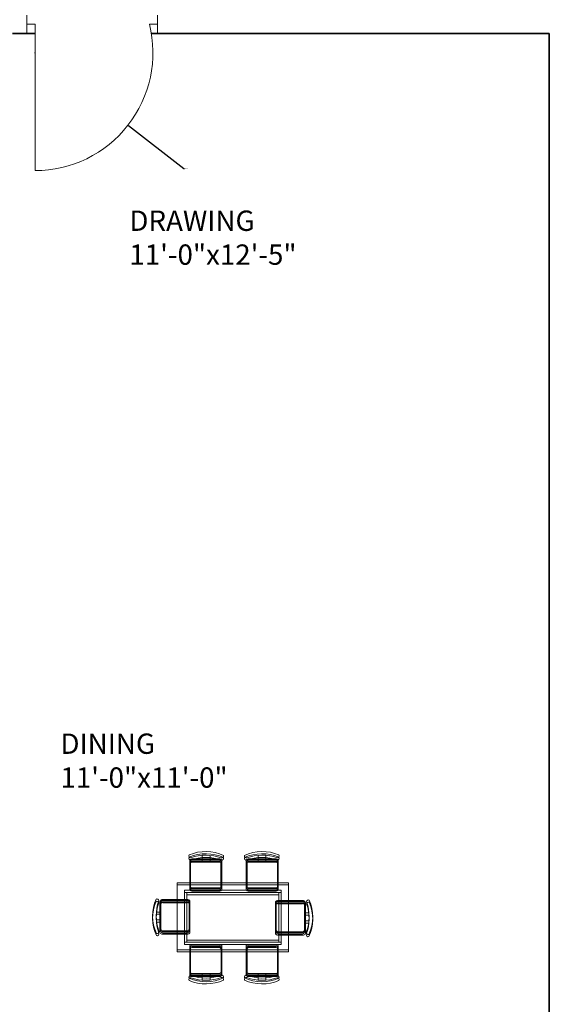
# Model space of a CAD drawing. Units: inches. Extents: x 2163 to 2982, y 1024 to 2288.
# Tile 4 of 22: x 2452 to 2582, y 1395 to 1637. Entities that reach past the tile are written whole.
import ezdxf

# ---------------------------------------------------------------- set-up
doc = ezdxf.new("R2010")
doc.units = ezdxf.units.IN
for name, color, linetype, lineweight in [('A-ANNO-DIMS', 2, 'Continuous', 18), ('A-AREA-IDEN', 7, 'Continuous', 18), ('A-DOOR', 11, 'Continuous', 18), ('A-FURN', 8, 'Continuous', 13), ('A-WALL', 7, 'Continuous', 35)]:
    doc.layers.add(name, color=color, linetype=linetype, lineweight=lineweight)
doc.styles.get("Standard").update_dxf_attribs({"font": 'arial.ttf'})
doc.dimstyles.get("Standard").update_dxf_attribs({"dimtxt": 0.18, "dimasz": 0.18, "dimexe": 0.18, "dimexo": 0.0625, "dimgap": 0.09, "dimtad": 0, "dimtih": 1, "dimtoh": 1, "dimdec": 4, "dimzin": 0, "dimdsep": 46, "dimtxsty": 'Standard', "dimcen": 0.09, "dimadec": 0, "dimazin": 0, "dimtfac": 1, "dimtdec": 4, "dimtofl": 0, "dimtmove": 0, "dimatfit": 3, "dimfxl": 1, "dimtolj": 1, "dimtzin": 0, "dimarcsym": 0})

# ---------------------------------------------------------------- blocks, each defined once
blk = doc.blocks.new('TABLE-DINING')
for points in [[(0, 17.02), (27.45, 17.02), (27.45, 0.55), (0, 0.55)], [(0, 17.02), (27.45, 17.02), (27.45, 0.55), (0, 0.55)], [(0, 17.02), (27.45, 17.02), (27.45, 0.55), (0, 0.55)], [(0, 17.02), (27.45, 17.02), (27.45, 0.55), (0, 0.55)], [(0, 16.47), (27.45, 16.47), (27.45, 0), (0, 0)], [(0, 16.47), (27.45, 16.47), (27.45, 0), (0, 0)], [(0, 16.47), (27.45, 16.47), (27.45, 0), (0, 0)], [(0, 16.47), (27.45, 16.47), (27.45, 0), (0, 0)], [(1.83, 15.19), (25.62, 15.19), (25.62, 2.38), (1.83, 2.38)], [(1.83, 15.19), (25.62, 15.19), (25.62, 2.38), (1.83, 2.38)], [(1.83, 15.19), (25.62, 15.19), (25.62, 2.38), (1.83, 2.38)], [(1.83, 15.19), (25.62, 15.19), (25.62, 2.38), (1.83, 2.38)], [(1.83, 14.64), (25.62, 14.64), (25.62, 1.83), (1.83, 1.83)], [(1.83, 14.64), (25.62, 14.64), (25.62, 1.83), (1.83, 1.83)], [(1.83, 14.64), (25.62, 14.64), (25.62, 1.83), (1.83, 1.83)], [(1.83, 14.64), (25.62, 14.64), (25.62, 1.83), (1.83, 1.83)], [(2.38, 14.64), (25.07, 14.64), (25.07, 2.93), (2.38, 2.93)], [(2.38, 14.64), (25.07, 14.64), (25.07, 2.93), (2.38, 2.93)], [(2.38, 14.64), (25.07, 14.64), (25.07, 2.93), (2.38, 2.93)], [(2.38, 14.64), (25.07, 14.64), (25.07, 2.93), (2.38, 2.93)], [(2.38, 14.09), (25.07, 14.09), (25.07, 2.38), (2.38, 2.38)], [(2.38, 14.09), (25.07, 14.09), (25.07, 2.38), (2.38, 2.38)], [(2.38, 14.09), (25.07, 14.09), (25.07, 2.38), (2.38, 2.38)], [(2.38, 14.09), (25.07, 14.09), (25.07, 2.38), (2.38, 2.38)]]:
    blk.add_lwpolyline(points, close=True)
blk = doc.blocks.new('CHAIR-DINING-A')
for points in [[(0.45, 8.2, -0.175809), (7.92, 8.14, 0.578392), (8.49, 8.77, 0.214524), (0.05, 8.88, 0.552014), (0.45, 8.2, -0.065079)], [(0.45, 8.2, -0.175809), (7.92, 8.14, 0.578392), (8.49, 8.77, 0.214524), (0.05, 8.88, 0.552014), (0.45, 8.2, -0.065079)], [(0.45, 8.2, -0.175809), (7.92, 8.14, 0.578392), (8.49, 8.77, 0.214524), (0.05, 8.88, 0.552014), (0.45, 8.2, -0.065079)], [(0.45, 8.2, -0.175809), (7.92, 8.14, 0.578392), (8.49, 8.77, 0.214524), (0.05, 8.88, 0.552014), (0.45, 8.2, -0.065079)], [(0.45, 7.65, -0.175809), (7.92, 7.6, 0.578392), (8.49, 8.22, 0.214524), (0.05, 8.33, 0.552014), (0.45, 7.65, -0.065079)], [(0.45, 7.65, -0.175809), (7.92, 7.6, 0.578392), (8.49, 8.22, 0.214524), (0.05, 8.33, 0.552014), (0.45, 7.65, -0.065079)], [(0.45, 7.65, -0.175809), (7.92, 7.6, 0.578392), (8.49, 8.22, 0.214524), (0.05, 8.33, 0.552014), (0.45, 7.65, -0.065079)], [(0.45, 7.65, -0.175809), (7.92, 7.6, 0.578392), (8.49, 8.22, 0.214524), (0.05, 8.33, 0.552014), (0.45, 7.65, -0.065079)], [(7.61, 7.9), (0.67, 7.9, 0.414214), (0.18, 7.42), (0.18, 1.03, 0.414214), (0.67, 0.55), (7.61, 0.55, 0.414214), (8.09, 1.03), (8.09, 7.42, 0.414214), (7.61, 7.9)], [(7.61, 7.9), (0.67, 7.9, 0.414214), (0.18, 7.42), (0.18, 1.03, 0.414214), (0.67, 0.55), (7.61, 0.55, 0.414214), (8.09, 1.03), (8.09, 7.42, 0.414214), (7.61, 7.9)], [(7.61, 7.9), (0.67, 7.9, 0.414214), (0.18, 7.42), (0.18, 1.03, 0.414214), (0.67, 0.55), (7.61, 0.55, 0.414214), (8.09, 1.03), (8.09, 7.42, 0.414214), (7.61, 7.9)], [(7.61, 7.9), (0.67, 7.9, 0.414214), (0.18, 7.42), (0.18, 1.03, 0.414214), (0.67, 0.55), (7.61, 0.55, 0.414214), (8.09, 1.03), (8.09, 7.42, 0.414214), (7.61, 7.9)], [(7.61, 7.35), (0.67, 7.35, 0.414214), (0.18, 6.87), (0.18, 0.49, 0.414214), (0.67, 0), (7.61, 0, 0.414214), (8.09, 0.49), (8.09, 6.87, 0.414214), (7.61, 7.35)], [(7.61, 7.35), (0.67, 7.35, 0.414214), (0.18, 6.87), (0.18, 0.49, 0.414214), (0.67, 0), (7.61, 0, 0.414214), (8.09, 0.49), (8.09, 6.87, 0.414214), (7.61, 7.35)], [(7.61, 7.35), (0.67, 7.35, 0.414214), (0.18, 6.87), (0.18, 0.49, 0.414214), (0.67, 0), (7.61, 0, 0.414214), (8.09, 0.49), (8.09, 6.87, 0.414214), (7.61, 7.35)], [(7.61, 7.35), (0.67, 7.35, 0.414214), (0.18, 6.87), (0.18, 0.49, 0.414214), (0.67, 0), (7.61, 0, 0.414214), (8.09, 0.49), (8.09, 6.87, 0.414214), (7.61, 7.35)], [(5.17, 7.9), (5.17, 8.78, -0.064759)], [(5.17, 7.9), (5.17, 8.78, -0.064759)], [(5.17, 7.9), (5.17, 8.78, -0.064759)], [(5.17, 7.9), (5.17, 8.78, -0.064759)], [(5.17, 7.35), (5.17, 8.23, -0.064759)], [(5.17, 7.35), (5.17, 8.23, -0.064759)], [(5.17, 7.35), (5.17, 8.23, -0.064759)], [(5.17, 7.35), (5.17, 8.23, -0.064759)]]:
    blk.add_lwpolyline(points, format="xyb")
for points in [[(0.67, 7.68), (7.39, 7.68, -0.414214), (7.87, 7.2), (7.87, 1.25, -0.414214), (7.39, 0.77), (0.67, 0.77, -0.512069), (0.4, 1.25), (0.4, 7.2, -0.512069)], [(0.67, 7.68), (7.39, 7.68, -0.414214), (7.87, 7.2), (7.87, 1.25, -0.414214), (7.39, 0.77), (0.67, 0.77, -0.512069), (0.4, 1.25), (0.4, 7.2, -0.512069)], [(0.67, 7.68), (7.39, 7.68, -0.414214), (7.87, 7.2), (7.87, 1.25, -0.414214), (7.39, 0.77), (0.67, 0.77, -0.512069), (0.4, 1.25), (0.4, 7.2, -0.512069)], [(0.67, 7.68), (7.39, 7.68, -0.414214), (7.87, 7.2), (7.87, 1.25, -0.414214), (7.39, 0.77), (0.67, 0.77, -0.512069), (0.4, 1.25), (0.4, 7.2, -0.512069)], [(0.67, 7.13), (7.39, 7.13, -0.414214), (7.87, 6.65), (7.87, 0.7, -0.414214), (7.39, 0.22), (0.67, 0.22, -0.512069), (0.4, 0.7), (0.4, 6.65, -0.512069)], [(0.67, 7.13), (7.39, 7.13, -0.414214), (7.87, 6.65), (7.87, 0.7, -0.414214), (7.39, 0.22), (0.67, 0.22, -0.512069), (0.4, 0.7), (0.4, 6.65, -0.512069)], [(0.67, 7.13), (7.39, 7.13, -0.414214), (7.87, 6.65), (7.87, 0.7, -0.414214), (7.39, 0.22), (0.67, 0.22, -0.512069), (0.4, 0.7), (0.4, 6.65, -0.512069)], [(0.67, 7.13), (7.39, 7.13, -0.414214), (7.87, 6.65), (7.87, 0.7, -0.414214), (7.39, 0.22), (0.67, 0.22, -0.512069), (0.4, 0.7), (0.4, 6.65, -0.512069)]]:
    blk.add_lwpolyline(points, format="xyb", close=True)
for points in [[(3.23, 8.8), (3.23, 7.9)], [(3.23, 8.8), (3.23, 7.9)], [(3.23, 8.79), (3.23, 7.9)], [(3.23, 8.79), (3.23, 7.9)], [(3.23, 8.25), (3.23, 7.35)], [(3.23, 8.25), (3.23, 7.35)], [(3.23, 8.25), (3.23, 7.35)], [(3.23, 8.25), (3.23, 7.35)]]:
    blk.add_lwpolyline(points)
blk = doc.blocks.new('*D43')
at = {"layer": 'A-ANNO-DIMS', "color": 0, "lineweight": -2, "transparency": 16777216}
for p, q in [((2455.83, 1628.97), (2456.01, 1628.97)), ((2455.92, 1628.88), (2455.92, 1629.06)), ((2492.45, 1600.48), (2478.89, 1611.05)), ((2492.63, 1600.48), (2492.45, 1600.48))]:
    blk.add_line(p, q, dxfattribs=at)
at = {"layer": 'A-ANNO-DIMS', "color": 0, "transparency": 16777216}
blk.add_solid([(2478.91, 1611.08), (2478.87, 1611.03), (2478.75, 1611.16)], dxfattribs=at)
at = {"layer": 'Defpoints', "color": 0, "transparency": 16777216}
for p in [(2455.92, 1628.97), (2478.75, 1611.16)]:
    blk.add_point(p, dxfattribs=at)
at = {"layer": 'A-ANNO-DIMS', "color": 0, "transparency": 16777216, "insert": (2493.11, 1600.48), "char_height": 0.18, "attachment_point": 5}
blk.add_mtext('\\A1;R28.95', dxfattribs=at)

msp = doc.modelspace()

# ---------------------------------------------------------------- linework, layer by layer
at = {"layer": 'A-DOOR'}
for p, q in [((2453.9219, 1633.7688), (2453.9219, 1638.2688)), ((2453.9219, 1638.2688), (2453.9219, 1636.0188)), ((2486.0038, 1638.2688), (2486.0038, 1633.7688)), ((2453.9219, 1636.0188), (2455.9219, 1636.0188)), ((2455.9219, 1636.0188), (2455.9219, 1600.0188)), ((2486.0038, 1636.0188), (2484.0038, 1636.0188)), ((2486.0038, 1633.7688), (2486.0038, 1636.0188))]:
    msp.add_line(p, q, dxfattribs=at)
msp.add_arc((2455.9219, 1628.9716), 28.9527, 270, 14.087641, dxfattribs=at)
at = {"layer": 'A-FURN'}
for points in [[(2507.9678, 1430.974, -0.57839206), (2507.4014, 1431.5967, -0.21452438), (2515.8396, 1431.7099, -0.55201397), (2515.4432, 1431.0306, 0.1758092), (2507.9678, 1430.974)], [(2507.9678, 1430.974, -0.57839206), (2507.4014, 1431.5967, -0.21452438), (2515.8396, 1431.7099, -0.55201397), (2515.4432, 1431.0306, 0.1758092), (2507.9678, 1430.974)], [(2507.9678, 1430.9737, -0.57839206), (2507.4015, 1431.5964, -0.21452438), (2515.8396, 1431.7096, -0.55201397), (2515.4432, 1431.0303, 0.1758092), (2507.9678, 1430.9737)], [(2507.9678, 1430.9737, -0.57839206), (2507.4015, 1431.5964, -0.21452438), (2515.8396, 1431.7096, -0.55201397), (2515.4432, 1431.0303, 0.1758092), (2507.9678, 1430.9737)], [(2507.9678, 1430.4251, -0.57839206), (2507.4014, 1431.0478, -0.21452438), (2515.8396, 1431.161, -0.55201397), (2515.4432, 1430.4817, 0.1758092), (2507.9678, 1430.4251)], [(2507.9678, 1430.4251, -0.57839206), (2507.4014, 1431.0478, -0.21452438), (2515.8396, 1431.161, -0.55201397), (2515.4432, 1430.4817, 0.1758092), (2507.9678, 1430.4251)], [(2507.9678, 1430.4248, -0.57839206), (2507.4015, 1431.0475, -0.21452438), (2515.8396, 1431.1607, -0.55201397), (2515.4432, 1430.4814, 0.1758092), (2507.9678, 1430.4248)], [(2507.9678, 1430.4248, -0.57839206), (2507.4015, 1431.0475, -0.21452438), (2515.8396, 1431.1607, -0.55201397), (2515.4432, 1430.4814, 0.1758092), (2507.9678, 1430.4248)], [(2510.7226, 1430.7306), (2510.7226, 1431.6082, 0.06475861)], [(2510.7226, 1430.7306), (2510.7226, 1431.6082, 0.06475861)], [(2510.7226, 1430.7303), (2510.7226, 1431.608, 0.06475861)], [(2510.7226, 1430.7303), (2510.7226, 1431.608, 0.06475861)], [(2515.2249, 1430.7306, -0.41421356), (2515.7104, 1430.245), (2515.7104, 1423.8639, -0.41421356), (2515.2249, 1423.3784), (2508.2849, 1423.3784, -0.41421356), (2507.7994, 1423.8639), (2507.7994, 1430.245, -0.41421356), (2508.2849, 1430.7306), (2515.2249, 1430.7306)], [(2515.2249, 1430.7306, -0.41421356), (2515.7104, 1430.245), (2515.7104, 1423.8639, -0.41421356), (2515.2249, 1423.3784), (2508.2849, 1423.3784, -0.41421356), (2507.7994, 1423.8639), (2507.7994, 1430.245, -0.41421356), (2508.2849, 1430.7306), (2515.2249, 1430.7306)], [(2515.2249, 1430.7303, -0.41421356), (2515.7104, 1430.2447), (2515.7104, 1423.8636, -0.41421356), (2515.2249, 1423.3781), (2508.2849, 1423.3781, -0.41421356), (2507.7994, 1423.8636), (2507.7994, 1430.2447, -0.41421356), (2508.2849, 1430.7303), (2515.2249, 1430.7303)], [(2515.2249, 1430.7303, -0.41421356), (2515.7104, 1430.2447), (2515.7104, 1423.8636, -0.41421356), (2515.2249, 1423.3781), (2508.2849, 1423.3781, -0.41421356), (2507.7994, 1423.8636), (2507.7994, 1430.2447, -0.41421356), (2508.2849, 1430.7303), (2515.2249, 1430.7303)], [(2515.2249, 1430.1816, -0.41421356), (2515.7104, 1429.6961), (2515.7104, 1423.315, -0.41421356), (2515.2249, 1422.8294), (2508.2849, 1422.8294, -0.41421356), (2507.7994, 1423.315), (2507.7994, 1429.6961, -0.41421356), (2508.2849, 1430.1816), (2515.2249, 1430.1816)], [(2515.2249, 1430.1816, -0.41421356), (2515.7104, 1429.6961), (2515.7104, 1423.315, -0.41421356), (2515.2249, 1422.8294), (2508.2849, 1422.8294, -0.41421356), (2507.7994, 1423.315), (2507.7994, 1429.6961, -0.41421356), (2508.2849, 1430.1816), (2515.2249, 1430.1816)], [(2515.2249, 1430.1814, -0.41421356), (2515.7104, 1429.6958), (2515.7104, 1423.3147, -0.41421356), (2515.2249, 1422.8292), (2508.2849, 1422.8292, -0.41421356), (2507.7994, 1423.3147), (2507.7994, 1429.6958, -0.41421356), (2508.2849, 1430.1814), (2515.2249, 1430.1814)], [(2515.2249, 1430.1814, -0.41421356), (2515.7104, 1429.6958), (2515.7104, 1423.3147, -0.41421356), (2515.2249, 1422.8292), (2508.2849, 1422.8292, -0.41421356), (2507.7994, 1423.3147), (2507.7994, 1429.6958, -0.41421356), (2508.2849, 1430.1814), (2515.2249, 1430.1814)], [(2510.7226, 1430.1816), (2510.7226, 1431.0593, 0.06475861)], [(2510.7226, 1430.1816), (2510.7226, 1431.0593, 0.06475861)], [(2510.7226, 1430.1814), (2510.7226, 1431.059, 0.06475861)], [(2510.7226, 1430.1814), (2510.7226, 1431.059, 0.06475861)], [(2486.3782, 1412.9785, -0.57839206), (2485.7555, 1412.4122, -0.21452438), (2485.6423, 1420.8504, -0.55201397), (2486.3216, 1420.454, 0.17580937), (2486.3782, 1412.9785)], [(2486.3782, 1412.9785, -0.57839206), (2485.7555, 1412.4122, -0.21452438), (2485.6423, 1420.8504, -0.55201397), (2486.3216, 1420.454, 0.17580937), (2486.3782, 1412.9785)], [(2486.3782, 1412.9782, -0.57839206), (2485.7555, 1412.4119, -0.21452438), (2485.6423, 1420.8501, -0.55201397), (2486.3216, 1420.4537, 0.17580937), (2486.3782, 1412.9782)], [(2486.3782, 1412.9782, -0.57839206), (2485.7555, 1412.4119, -0.21452438), (2485.6423, 1420.8501, -0.55201397), (2486.3216, 1420.4537, 0.17580937), (2486.3782, 1412.9782)], [(2486.3782, 1412.4296, -0.57839206), (2485.7555, 1411.8633, -0.21452438), (2485.6423, 1420.3015, -0.55201397), (2486.3216, 1419.9051, 0.17580937), (2486.3782, 1412.4296)], [(2486.3782, 1412.4296, -0.57839206), (2485.7555, 1411.8633, -0.21452438), (2485.6423, 1420.3015, -0.55201397), (2486.3216, 1419.9051, 0.17580937), (2486.3782, 1412.4296)], [(2486.3782, 1412.4293, -0.57839206), (2485.7555, 1411.863, -0.21452438), (2485.6423, 1420.3012, -0.55201397), (2486.3216, 1419.9048, 0.17580937), (2486.3782, 1412.4293)], [(2486.3782, 1412.4293, -0.57839206), (2485.7555, 1411.863, -0.21452438), (2485.6423, 1420.3012, -0.55201397), (2486.3216, 1419.9048, 0.17580937), (2486.3782, 1412.4293)], [(2486.6217, 1420.2356, -0.41421356), (2487.1072, 1420.7212), (2493.4883, 1420.7212, -0.41421356), (2493.9739, 1420.2356), (2493.9739, 1413.2957, -0.41421356), (2493.4883, 1412.8102), (2487.1072, 1412.8102, -0.41421356), (2486.6217, 1413.2957), (2486.6217, 1420.2356)], [(2486.6217, 1420.2356, -0.41421356), (2487.1072, 1420.7212), (2493.4883, 1420.7212, -0.41421356), (2493.9739, 1420.2356), (2493.9739, 1413.2957, -0.41421356), (2493.4883, 1412.8102), (2487.1072, 1412.8102, -0.41421356), (2486.6217, 1413.2957), (2486.6217, 1420.2356)], [(2486.6217, 1420.2353, -0.41421356), (2487.1072, 1420.7209), (2493.4883, 1420.7209, -0.41421356), (2493.9739, 1420.2353), (2493.9739, 1413.2954, -0.41421356), (2493.4883, 1412.8099), (2487.1072, 1412.8099, -0.41421356), (2486.6217, 1413.2954), (2486.6217, 1420.2353)], [(2486.6217, 1420.2353, -0.41421356), (2487.1072, 1420.7209), (2493.4883, 1420.7209, -0.41421356), (2493.9739, 1420.2353), (2493.9739, 1413.2954, -0.41421356), (2493.4883, 1412.8099), (2487.1072, 1412.8099, -0.41421356), (2486.6217, 1413.2954), (2486.6217, 1420.2353)], [(2486.6217, 1419.6867, -0.41421356), (2487.1072, 1420.1722), (2493.4883, 1420.1722, -0.41421356), (2493.9739, 1419.6867), (2493.9739, 1412.7468, -0.41421356), (2493.4883, 1412.2612), (2487.1072, 1412.2612, -0.41421356), (2486.6217, 1412.7468), (2486.6217, 1419.6867)], [(2486.6217, 1419.6867, -0.41421356), (2487.1072, 1420.1722), (2493.4883, 1420.1722, -0.41421356), (2493.9739, 1419.6867), (2493.9739, 1412.7468, -0.41421356), (2493.4883, 1412.2612), (2487.1072, 1412.2612, -0.41421356), (2486.6217, 1412.7468), (2486.6217, 1419.6867)], [(2486.6217, 1419.6864, -0.41421356), (2487.1072, 1420.172), (2493.4883, 1420.172, -0.41421356), (2493.9739, 1419.6864), (2493.9739, 1412.7465, -0.41421356), (2493.4883, 1412.261), (2487.1072, 1412.261, -0.41421356), (2486.6217, 1412.7465), (2486.6217, 1419.6864)], [(2486.6217, 1419.6864, -0.41421356), (2487.1072, 1420.172), (2493.4883, 1420.172, -0.41421356), (2493.9739, 1419.6864), (2493.9739, 1412.7465, -0.41421356), (2493.4883, 1412.261), (2487.1072, 1412.261, -0.41421356), (2486.6217, 1412.7465), (2486.6217, 1419.6864)], [(2522.3591, 1419.998, 0.41421356), (2521.8736, 1420.4835), (2515.4924, 1420.4835, 0.41421356), (2515.0069, 1419.998), (2515.0069, 1413.058, 0.41421356), (2515.4924, 1412.5725), (2521.8736, 1412.5725, 0.41421356), (2522.3591, 1413.058), (2522.3591, 1419.998)], [(2522.3591, 1419.998, 0.41421356), (2521.8736, 1420.4835), (2515.4924, 1420.4835, 0.41421356), (2515.0069, 1419.998), (2515.0069, 1413.058, 0.41421356), (2515.4924, 1412.5725), (2521.8736, 1412.5725, 0.41421356), (2522.3591, 1413.058), (2522.3591, 1419.998)], [(2522.3591, 1419.9977, 0.41421356), (2521.8736, 1420.4832), (2515.4925, 1420.4832, 0.41421356), (2515.0069, 1419.9977), (2515.0069, 1413.0577, 0.41421356), (2515.4925, 1412.5722), (2521.8736, 1412.5722, 0.41421356), (2522.3591, 1413.0577), (2522.3591, 1419.9977)], [(2522.3591, 1419.9977, 0.41421356), (2521.8736, 1420.4832), (2515.4925, 1420.4832, 0.41421356), (2515.0069, 1419.9977), (2515.0069, 1413.0577, 0.41421356), (2515.4925, 1412.5722), (2521.8736, 1412.5722, 0.41421356), (2522.3591, 1413.0577), (2522.3591, 1419.9977)], [(2522.3591, 1419.449, 0.41421356), (2521.8736, 1419.9346), (2515.4924, 1419.9346, 0.41421356), (2515.0069, 1419.449), (2515.0069, 1412.5091, 0.41421356), (2515.4924, 1412.0236), (2521.8736, 1412.0236, 0.41421356), (2522.3591, 1412.5091), (2522.3591, 1419.449)], [(2522.3591, 1419.449, 0.41421356), (2521.8736, 1419.9346), (2515.4924, 1419.9346, 0.41421356), (2515.0069, 1419.449), (2515.0069, 1412.5091, 0.41421356), (2515.4924, 1412.0236), (2521.8736, 1412.0236, 0.41421356), (2522.3591, 1412.5091), (2522.3591, 1419.449)], [(2522.3591, 1419.4487, 0.41421356), (2521.8736, 1419.9343), (2515.4925, 1419.9343, 0.41421356), (2515.0069, 1419.4487), (2515.0069, 1412.5088, 0.41421356), (2515.4925, 1412.0233), (2521.8736, 1412.0233, 0.41421356), (2522.3591, 1412.5088), (2522.3591, 1419.4487)], [(2522.3591, 1419.4487, 0.41421356), (2521.8736, 1419.9343), (2515.4925, 1419.9343, 0.41421356), (2515.0069, 1419.4487), (2515.0069, 1412.5088, 0.41421356), (2515.4925, 1412.0233), (2521.8736, 1412.0233, 0.41421356), (2522.3591, 1412.5088), (2522.3591, 1419.4487)], [(2522.6591, 1420.2163, -0.17580919), (2522.6025, 1412.7409, 0.57839206), (2523.2252, 1412.1745, 0.21452438), (2523.3385, 1420.6127, 0.55201397), (2522.6591, 1420.2163, -0.06507904)], [(2522.6591, 1420.2163, -0.17580919), (2522.6025, 1412.7409, 0.57839206), (2523.2252, 1412.1745, 0.21452438), (2523.3385, 1420.6127, 0.55201397), (2522.6591, 1420.2163, -0.06507904)], [(2522.6592, 1420.216, -0.17580919), (2522.6025, 1412.7406, 0.57839206), (2523.2253, 1412.1742, 0.21452438), (2523.3385, 1420.6124, 0.55201397), (2522.6592, 1420.216, -0.06507904)], [(2522.6592, 1420.216, -0.17580919), (2522.6025, 1412.7406, 0.57839206), (2523.2253, 1412.1742, 0.21452438), (2523.3385, 1420.6124, 0.55201397), (2522.6592, 1420.216, -0.06507904)], [(2522.6591, 1419.6674, -0.17580919), (2522.6025, 1412.1919, 0.57839206), (2523.2252, 1411.6256, 0.21452438), (2523.3385, 1420.0638, 0.55201397), (2522.6591, 1419.6674, -0.06507904)], [(2522.6591, 1419.6674, -0.17580919), (2522.6025, 1412.1919, 0.57839206), (2523.2252, 1411.6256, 0.21452438), (2523.3385, 1420.0638, 0.55201397), (2522.6591, 1419.6674, -0.06507904)], [(2522.6592, 1419.6671, -0.17580919), (2522.6025, 1412.1917, 0.57839206), (2523.2253, 1411.6253, 0.21452438), (2523.3385, 1420.0635, 0.55201397), (2522.6592, 1419.6671, -0.06507904)], [(2522.6592, 1419.6671, -0.17580919), (2522.6025, 1412.1917, 0.57839206), (2523.2253, 1411.6253, 0.21452438), (2523.3385, 1420.0635, 0.55201397), (2522.6592, 1419.6671, -0.06507904)], [(2486.6217, 1415.7333), (2485.744, 1415.7333, 0.06475861)], [(2486.6217, 1415.7333), (2485.744, 1415.7333, 0.06475861)], [(2486.6217, 1415.7331), (2485.744, 1415.7331, 0.06475861)], [(2486.6217, 1415.7331), (2485.744, 1415.7331, 0.06475861)], [(2486.6217, 1415.1844), (2485.744, 1415.1844, 0.06475861)], [(2486.6217, 1415.1844), (2485.744, 1415.1844, 0.06475861)], [(2486.6217, 1415.1841), (2485.744, 1415.1841, 0.06475861)], [(2486.6217, 1415.1841), (2485.744, 1415.1841, 0.06475861)], [(2522.3591, 1415.4957), (2523.2368, 1415.4957, -0.06475861)], [(2522.3591, 1415.4957), (2523.2368, 1415.4957, -0.06475861)], [(2522.3591, 1415.4954), (2523.2368, 1415.4954, -0.06475861)], [(2522.3591, 1415.4954), (2523.2368, 1415.4954, -0.06475861)], [(2522.3591, 1414.9468), (2523.2368, 1414.9468, -0.06475861)], [(2522.3591, 1414.9468), (2523.2368, 1414.9468, -0.06475861)], [(2522.3591, 1414.9465), (2523.2368, 1414.9465, -0.06475861)], [(2522.3591, 1414.9465), (2523.2368, 1414.9465, -0.06475861)], [(2501.3573, 1402.3648), (2494.4173, 1402.3648, -0.41421356), (2493.9318, 1402.8503), (2493.9318, 1409.2315, -0.41421356), (2494.4173, 1409.717), (2501.3573, 1409.717, -0.41421356), (2501.8428, 1409.2315), (2501.8428, 1402.8503, -0.41421356), (2501.3573, 1402.3648)], [(2501.3573, 1402.3648), (2494.4173, 1402.3648, -0.41421356), (2493.9318, 1402.8503), (2493.9318, 1409.2315, -0.41421356), (2494.4173, 1409.717), (2501.3573, 1409.717, -0.41421356), (2501.8428, 1409.2315), (2501.8428, 1402.8503, -0.41421356), (2501.3573, 1402.3648)], [(2501.3573, 1402.3645), (2494.4173, 1402.3645, -0.41421356), (2493.9318, 1402.85), (2493.9318, 1409.2312, -0.41421356), (2494.4173, 1409.7167), (2501.3573, 1409.7167, -0.41421356), (2501.8428, 1409.2312), (2501.8428, 1402.85, -0.41421356), (2501.3573, 1402.3645)], [(2501.3573, 1402.3645), (2494.4173, 1402.3645, -0.41421356), (2493.9318, 1402.85), (2493.9318, 1409.2312, -0.41421356), (2494.4173, 1409.7167), (2501.3573, 1409.7167, -0.41421356), (2501.8428, 1409.2312), (2501.8428, 1402.85, -0.41421356), (2501.3573, 1402.3645)], [(2515.2249, 1402.3648, 0.41421356), (2515.7104, 1402.8503), (2515.7104, 1409.2315, 0.41421356), (2515.2249, 1409.717), (2508.2849, 1409.717, 0.41421356), (2507.7994, 1409.2315), (2507.7994, 1402.8503, 0.41421356), (2508.2849, 1402.3648), (2515.2249, 1402.3648)], [(2515.2249, 1402.3648, 0.41421356), (2515.7104, 1402.8503), (2515.7104, 1409.2315, 0.41421356), (2515.2249, 1409.717), (2508.2849, 1409.717, 0.41421356), (2507.7994, 1409.2315), (2507.7994, 1402.8503, 0.41421356), (2508.2849, 1402.3648), (2515.2249, 1402.3648)], [(2515.2249, 1402.3645, 0.41421356), (2515.7104, 1402.85), (2515.7104, 1409.2312, 0.41421356), (2515.2249, 1409.7167), (2508.2849, 1409.7167, 0.41421356), (2507.7994, 1409.2312), (2507.7994, 1402.85, 0.41421356), (2508.2849, 1402.3645), (2515.2249, 1402.3645)], [(2515.2249, 1402.3645, 0.41421356), (2515.7104, 1402.85), (2515.7104, 1409.2312, 0.41421356), (2515.2249, 1409.7167), (2508.2849, 1409.7167, 0.41421356), (2507.7994, 1409.2312), (2507.7994, 1402.85, 0.41421356), (2508.2849, 1402.3645), (2515.2249, 1402.3645)], [(2501.3573, 1401.8159), (2494.4173, 1401.8159, -0.41421356), (2493.9318, 1402.3014), (2493.9318, 1408.6826, -0.41421356), (2494.4173, 1409.1681), (2501.3573, 1409.1681, -0.41421356), (2501.8428, 1408.6826), (2501.8428, 1402.3014, -0.41421356), (2501.3573, 1401.8159)], [(2501.3573, 1401.8159), (2494.4173, 1401.8159, -0.41421356), (2493.9318, 1402.3014), (2493.9318, 1408.6826, -0.41421356), (2494.4173, 1409.1681), (2501.3573, 1409.1681, -0.41421356), (2501.8428, 1408.6826), (2501.8428, 1402.3014, -0.41421356), (2501.3573, 1401.8159)], [(2501.3573, 1401.8156), (2494.4173, 1401.8156, -0.41421356), (2493.9318, 1402.3011), (2493.9318, 1408.6823, -0.41421356), (2494.4173, 1409.1678), (2501.3573, 1409.1678, -0.41421356), (2501.8428, 1408.6823), (2501.8428, 1402.3011, -0.41421356), (2501.3573, 1401.8156)], [(2501.3573, 1401.8156), (2494.4173, 1401.8156, -0.41421356), (2493.9318, 1402.3011), (2493.9318, 1408.6823, -0.41421356), (2494.4173, 1409.1678), (2501.3573, 1409.1678, -0.41421356), (2501.8428, 1408.6823), (2501.8428, 1402.3011, -0.41421356), (2501.3573, 1401.8156)], [(2515.2249, 1401.8159, 0.41421356), (2515.7104, 1402.3014), (2515.7104, 1408.6826, 0.41421356), (2515.2249, 1409.1681), (2508.2849, 1409.1681, 0.41421356), (2507.7994, 1408.6826), (2507.7994, 1402.3014, 0.41421356), (2508.2849, 1401.8159), (2515.2249, 1401.8159)], [(2515.2249, 1401.8159, 0.41421356), (2515.7104, 1402.3014), (2515.7104, 1408.6826, 0.41421356), (2515.2249, 1409.1681), (2508.2849, 1409.1681, 0.41421356), (2507.7994, 1408.6826), (2507.7994, 1402.3014, 0.41421356), (2508.2849, 1401.8159), (2515.2249, 1401.8159)], [(2515.2249, 1401.8156, 0.41421356), (2515.7104, 1402.3011), (2515.7104, 1408.6823, 0.41421356), (2515.2249, 1409.1678), (2508.2849, 1409.1678, 0.41421356), (2507.7994, 1408.6823), (2507.7994, 1402.3011, 0.41421356), (2508.2849, 1401.8156), (2515.2249, 1401.8156)], [(2515.2249, 1401.8156, 0.41421356), (2515.7104, 1402.3011), (2515.7104, 1408.6823, 0.41421356), (2515.2249, 1409.1678), (2508.2849, 1409.1678, 0.41421356), (2507.7994, 1408.6823), (2507.7994, 1402.3011, 0.41421356), (2508.2849, 1401.8156), (2515.2249, 1401.8156)], [(2498.9196, 1402.3648), (2498.9196, 1401.4871, 0.06475861)], [(2498.9196, 1402.3648), (2498.9196, 1401.4871, 0.06475861)], [(2498.9196, 1402.3645), (2498.9196, 1401.4868, 0.06475861)], [(2498.9196, 1402.3645), (2498.9196, 1401.4868, 0.06475861)], [(2510.7226, 1402.3648), (2510.7226, 1401.4871, -0.06475861)], [(2510.7226, 1402.3648), (2510.7226, 1401.4871, -0.06475861)], [(2510.7226, 1402.3645), (2510.7226, 1401.4868, -0.06475861)], [(2510.7226, 1402.3645), (2510.7226, 1401.4868, -0.06475861)], [(2501.6744, 1402.1214, -0.57839206), (2502.2407, 1401.4987, -0.21452438), (2493.8026, 1401.3855, -0.55201397), (2494.199, 1402.0648, 0.17580929), (2501.6744, 1402.1214)], [(2501.6744, 1402.1214, -0.57839206), (2502.2407, 1401.4987, -0.21452438), (2493.8026, 1401.3855, -0.55201397), (2494.199, 1402.0648, 0.17580929), (2501.6744, 1402.1214)], [(2501.6744, 1402.1211, -0.57839206), (2502.2408, 1401.4984, -0.21452438), (2493.8026, 1401.3852, -0.55201397), (2494.199, 1402.0645, 0.17580929), (2501.6744, 1402.1211)], [(2501.6744, 1402.1211, -0.57839206), (2502.2408, 1401.4984, -0.21452438), (2493.8026, 1401.3852, -0.55201397), (2494.199, 1402.0645, 0.17580929), (2501.6744, 1402.1211)], [(2501.6744, 1401.5725, -0.57839206), (2502.2407, 1400.9498, -0.21452438), (2493.8026, 1400.8365, -0.55201397), (2494.199, 1401.5159, 0.17580929), (2501.6744, 1401.5725)], [(2501.6744, 1401.5725, -0.57839206), (2502.2407, 1400.9498, -0.21452438), (2493.8026, 1400.8365, -0.55201397), (2494.199, 1401.5159, 0.17580929), (2501.6744, 1401.5725)], [(2501.6744, 1401.5722, -0.57839206), (2502.2408, 1400.9495, -0.21452438), (2493.8026, 1400.8362, -0.55201397), (2494.199, 1401.5156, 0.17580929), (2501.6744, 1401.5722)], [(2501.6744, 1401.5722, -0.57839206), (2502.2408, 1400.9495, -0.21452438), (2493.8026, 1400.8362, -0.55201397), (2494.199, 1401.5156, 0.17580929), (2501.6744, 1401.5722)], [(2498.9196, 1401.8159), (2498.9196, 1400.9382, 0.06475861)], [(2498.9196, 1401.8159), (2498.9196, 1400.9382, 0.06475861)], [(2498.9196, 1401.8156), (2498.9196, 1400.9379, 0.06475861)], [(2498.9196, 1401.8156), (2498.9196, 1400.9379, 0.06475861)], [(2515.4432, 1402.0648, -0.17580928), (2507.9678, 1402.1214, 0.57839206), (2507.4014, 1401.4987, 0.21452438), (2515.8396, 1401.3855, 0.55201397), (2515.4432, 1402.0648, -0.06507904)], [(2515.4432, 1402.0648, -0.17580928), (2507.9678, 1402.1214, 0.57839206), (2507.4014, 1401.4987, 0.21452438), (2515.8396, 1401.3855, 0.55201397), (2515.4432, 1402.0648, -0.06507904)], [(2515.4432, 1402.0645, -0.17580928), (2507.9678, 1402.1211, 0.57839206), (2507.4015, 1401.4984, 0.21452438), (2515.8396, 1401.3852, 0.55201397), (2515.4432, 1402.0645, -0.06507904)], [(2515.4432, 1402.0645, -0.17580928), (2507.9678, 1402.1211, 0.57839206), (2507.4015, 1401.4984, 0.21452438), (2515.8396, 1401.3852, 0.55201397), (2515.4432, 1402.0645, -0.06507904)], [(2515.4432, 1401.5159, -0.17580928), (2507.9678, 1401.5725, 0.57839206), (2507.4014, 1400.9498, 0.21452438), (2515.8396, 1400.8365, 0.55201397), (2515.4432, 1401.5159, -0.06507904)], [(2515.4432, 1401.5159, -0.17580928), (2507.9678, 1401.5725, 0.57839206), (2507.4014, 1400.9498, 0.21452438), (2515.8396, 1400.8365, 0.55201397), (2515.4432, 1401.5159, -0.06507904)], [(2515.4432, 1401.5156, -0.17580928), (2507.9678, 1401.5722, 0.57839206), (2507.4015, 1400.9495, 0.21452438), (2515.8396, 1400.8362, 0.55201397), (2515.4432, 1401.5156, -0.06507904)], [(2515.4432, 1401.5156, -0.17580928), (2507.9678, 1401.5722, 0.57839206), (2507.4015, 1400.9495, 0.21452438), (2515.8396, 1400.8362, 0.55201397), (2515.4432, 1401.5156, -0.06507904)], [(2510.7226, 1401.8159), (2510.7226, 1400.9382, -0.06475861)], [(2510.7226, 1401.8159), (2510.7226, 1400.9382, -0.06475861)], [(2510.7226, 1401.8156), (2510.7226, 1400.9379, -0.06475861)], [(2510.7226, 1401.8156), (2510.7226, 1400.9379, -0.06475861)]]:
    msp.add_lwpolyline(points, format="xyb", dxfattribs=at)
for points in [[(2512.6652, 1431.6242), (2512.6652, 1430.7306)], [(2512.6652, 1431.6242), (2512.6652, 1430.7306)], [(2512.6652, 1431.6239), (2512.6652, 1430.7303)], [(2512.6652, 1431.6239), (2512.6652, 1430.7303)], [(2512.6652, 1431.0753), (2512.6652, 1430.1816)], [(2512.6652, 1431.0753), (2512.6652, 1430.1816)], [(2512.6652, 1431.075), (2512.6652, 1430.1814)], [(2512.6652, 1431.075), (2512.6652, 1430.1814)], [(2485.728, 1417.6759), (2486.6217, 1417.6759)], [(2485.728, 1417.6759), (2486.6217, 1417.6759)], [(2485.728, 1417.6756), (2486.6217, 1417.6756)], [(2485.728, 1417.6756), (2486.6217, 1417.6756)], [(2485.728, 1417.127), (2486.6217, 1417.127)], [(2485.728, 1417.127), (2486.6217, 1417.127)], [(2485.728, 1417.1267), (2486.6217, 1417.1267)], [(2485.728, 1417.1267), (2486.6217, 1417.1267)], [(2523.2528, 1417.4383), (2522.3591, 1417.4383)], [(2523.2528, 1417.4383), (2522.3591, 1417.4383)], [(2523.2528, 1417.438), (2522.3591, 1417.438)], [(2523.2528, 1417.438), (2522.3591, 1417.438)], [(2523.2528, 1416.8893), (2522.3591, 1416.8893)], [(2523.2528, 1416.8893), (2522.3591, 1416.8893)], [(2523.2528, 1416.8891), (2522.3591, 1416.8891)], [(2523.2528, 1416.8891), (2522.3591, 1416.8891)], [(2496.977, 1401.4712), (2496.977, 1402.3648)], [(2496.977, 1401.4712), (2496.977, 1402.3648)], [(2496.977, 1401.4709), (2496.977, 1402.3645)], [(2496.977, 1401.4709), (2496.977, 1402.3645)], [(2512.6652, 1401.4712), (2512.6652, 1402.3648)], [(2512.6652, 1401.4712), (2512.6652, 1402.3648)], [(2512.6652, 1401.4709), (2512.6652, 1402.3645)], [(2512.6652, 1401.4709), (2512.6652, 1402.3645)], [(2496.977, 1400.9223), (2496.977, 1401.8159)], [(2496.977, 1400.9223), (2496.977, 1401.8159)], [(2496.977, 1400.922), (2496.977, 1401.8156)], [(2496.977, 1400.922), (2496.977, 1401.8156)], [(2512.6652, 1400.9223), (2512.6652, 1401.8159)], [(2512.6652, 1400.9223), (2512.6652, 1401.8159)], [(2512.6652, 1400.922), (2512.6652, 1401.8156)], [(2512.6652, 1400.922), (2512.6652, 1401.8156)]]:
    msp.add_lwpolyline(points, dxfattribs=at)
for points in [[(2515.2219, 1430.5118), (2508.5037, 1430.5118, 0.41421356), (2508.0181, 1430.0263), (2508.0181, 1424.0826, 0.41421356), (2508.5037, 1423.5971), (2515.2219, 1423.5971, 0.51206948), (2515.4917, 1424.0826), (2515.4917, 1430.0263, 0.51206948)], [(2515.2219, 1430.5118), (2508.5037, 1430.5118, 0.41421356), (2508.0181, 1430.0263), (2508.0181, 1424.0826, 0.41421356), (2508.5037, 1423.5971), (2515.2219, 1423.5971, 0.51206948), (2515.4917, 1424.0826), (2515.4917, 1430.0263, 0.51206948)], [(2515.2219, 1430.5115), (2508.5037, 1430.5115, 0.41421356), (2508.0181, 1430.026), (2508.0181, 1424.0823, 0.41421356), (2508.5037, 1423.5968), (2515.2219, 1423.5968, 0.51206948), (2515.4917, 1424.0823), (2515.4917, 1430.026, 0.51206948)], [(2515.2219, 1430.5115), (2508.5037, 1430.5115, 0.41421356), (2508.0181, 1430.026), (2508.0181, 1424.0823, 0.41421356), (2508.5037, 1423.5968), (2515.2219, 1423.5968, 0.51206948), (2515.4917, 1424.0823), (2515.4917, 1430.026, 0.51206948)], [(2515.2219, 1429.9629), (2508.5037, 1429.9629, 0.41421356), (2508.0181, 1429.4774), (2508.0181, 1423.5337, 0.41421356), (2508.5037, 1423.0482), (2515.2219, 1423.0482, 0.51206948), (2515.4917, 1423.5337), (2515.4917, 1429.4774, 0.51206948)], [(2515.2219, 1429.9629), (2508.5037, 1429.9629, 0.41421356), (2508.0181, 1429.4774), (2508.0181, 1423.5337, 0.41421356), (2508.5037, 1423.0482), (2515.2219, 1423.0482, 0.51206948), (2515.4917, 1423.5337), (2515.4917, 1429.4774, 0.51206948)], [(2515.2219, 1429.9626), (2508.5037, 1429.9626, 0.41421356), (2508.0181, 1429.4771), (2508.0181, 1423.5334, 0.41421356), (2508.5037, 1423.0479), (2515.2219, 1423.0479, 0.51206948), (2515.4917, 1423.5334), (2515.4917, 1429.4771, 0.51206948)], [(2515.2219, 1429.9626), (2508.5037, 1429.9626, 0.41421356), (2508.0181, 1429.4771), (2508.0181, 1423.5334, 0.41421356), (2508.5037, 1423.0479), (2515.2219, 1423.0479, 0.51206948), (2515.4917, 1423.5334), (2515.4917, 1429.4771, 0.51206948)], [(2486.8404, 1420.2327), (2486.8404, 1413.5144, 0.41421356), (2487.3259, 1413.0289), (2493.2696, 1413.0289, 0.41421356), (2493.7551, 1413.5144), (2493.7551, 1420.2327, 0.51206948), (2493.2696, 1420.5024), (2487.3259, 1420.5024, 0.51206948)], [(2486.8404, 1420.2327), (2486.8404, 1413.5144, 0.41421356), (2487.3259, 1413.0289), (2493.2696, 1413.0289, 0.41421356), (2493.7551, 1413.5144), (2493.7551, 1420.2327, 0.51206948), (2493.2696, 1420.5024), (2487.3259, 1420.5024, 0.51206948)], [(2486.8404, 1420.2324), (2486.8404, 1413.5141, 0.41421356), (2487.3259, 1413.0286), (2493.2696, 1413.0286, 0.41421356), (2493.7551, 1413.5141), (2493.7551, 1420.2324, 0.51206948), (2493.2696, 1420.5021), (2487.3259, 1420.5021, 0.51206948)], [(2486.8404, 1420.2324), (2486.8404, 1413.5141, 0.41421356), (2487.3259, 1413.0286), (2493.2696, 1413.0286, 0.41421356), (2493.7551, 1413.5141), (2493.7551, 1420.2324, 0.51206948), (2493.2696, 1420.5021), (2487.3259, 1420.5021, 0.51206948)], [(2486.8404, 1419.6838), (2486.8404, 1412.9655, 0.41421356), (2487.3259, 1412.48), (2493.2696, 1412.48, 0.41421356), (2493.7551, 1412.9655), (2493.7551, 1419.6838, 0.51206948), (2493.2696, 1419.9535), (2487.3259, 1419.9535, 0.51206948)], [(2486.8404, 1419.6838), (2486.8404, 1412.9655, 0.41421356), (2487.3259, 1412.48), (2493.2696, 1412.48, 0.41421356), (2493.7551, 1412.9655), (2493.7551, 1419.6838, 0.51206948), (2493.2696, 1419.9535), (2487.3259, 1419.9535, 0.51206948)], [(2486.8404, 1419.6835), (2486.8404, 1412.9652, 0.41421356), (2487.3259, 1412.4797), (2493.2696, 1412.4797, 0.41421356), (2493.7551, 1412.9652), (2493.7551, 1419.6835, 0.51206948), (2493.2696, 1419.9532), (2487.3259, 1419.9532, 0.51206948)], [(2486.8404, 1419.6835), (2486.8404, 1412.9652, 0.41421356), (2487.3259, 1412.4797), (2493.2696, 1412.4797, 0.41421356), (2493.7551, 1412.9652), (2493.7551, 1419.6835, 0.51206948), (2493.2696, 1419.9532), (2487.3259, 1419.9532, 0.51206948)], [(2522.1404, 1419.995), (2522.1404, 1413.2767, -0.41421356), (2521.6549, 1412.7912), (2515.7112, 1412.7912, -0.41421356), (2515.2257, 1413.2767), (2515.2257, 1419.995, -0.51206948), (2515.7112, 1420.2647), (2521.6549, 1420.2647, -0.51206948)], [(2522.1404, 1419.995), (2522.1404, 1413.2767, -0.41421356), (2521.6549, 1412.7912), (2515.7112, 1412.7912, -0.41421356), (2515.2257, 1413.2767), (2515.2257, 1419.995, -0.51206948), (2515.7112, 1420.2647), (2521.6549, 1420.2647, -0.51206948)], [(2522.1404, 1419.9947), (2522.1404, 1413.2765, -0.41421356), (2521.6549, 1412.7909), (2515.7112, 1412.7909, -0.41421356), (2515.2257, 1413.2765), (2515.2257, 1419.9947, -0.51206948), (2515.7112, 1420.2645), (2521.6549, 1420.2645, -0.51206948)], [(2522.1404, 1419.9947), (2522.1404, 1413.2765, -0.41421356), (2521.6549, 1412.7909), (2515.7112, 1412.7909, -0.41421356), (2515.2257, 1413.2765), (2515.2257, 1419.9947, -0.51206948), (2515.7112, 1420.2645), (2521.6549, 1420.2645, -0.51206948)], [(2522.1404, 1419.4461), (2522.1404, 1412.7278, -0.41421356), (2521.6549, 1412.2423), (2515.7112, 1412.2423, -0.41421356), (2515.2257, 1412.7278), (2515.2257, 1419.4461, -0.51206948), (2515.7112, 1419.7158), (2521.6549, 1419.7158, -0.51206948)], [(2522.1404, 1419.4461), (2522.1404, 1412.7278, -0.41421356), (2521.6549, 1412.2423), (2515.7112, 1412.2423, -0.41421356), (2515.2257, 1412.7278), (2515.2257, 1419.4461, -0.51206948), (2515.7112, 1419.7158), (2521.6549, 1419.7158, -0.51206948)], [(2522.1404, 1419.4458), (2522.1404, 1412.7275, -0.41421356), (2521.6549, 1412.242), (2515.7112, 1412.242, -0.41421356), (2515.2257, 1412.7275), (2515.2257, 1419.4458, -0.51206948), (2515.7112, 1419.7155), (2521.6549, 1419.7155, -0.51206948)], [(2522.1404, 1419.4458), (2522.1404, 1412.7275, -0.41421356), (2521.6549, 1412.242), (2515.7112, 1412.242, -0.41421356), (2515.2257, 1412.7275), (2515.2257, 1419.4458, -0.51206948), (2515.7112, 1419.7155), (2521.6549, 1419.7155, -0.51206948)], [(2494.4203, 1402.5835), (2501.1385, 1402.5835, 0.41421356), (2501.6241, 1403.0691), (2501.6241, 1409.0127, 0.41421356), (2501.1385, 1409.4983), (2494.4203, 1409.4983, 0.51206948), (2494.1505, 1409.0127), (2494.1505, 1403.0691, 0.51206948)], [(2494.4203, 1402.5835), (2501.1385, 1402.5835, 0.41421356), (2501.6241, 1403.0691), (2501.6241, 1409.0127, 0.41421356), (2501.1385, 1409.4983), (2494.4203, 1409.4983, 0.51206948), (2494.1505, 1409.0127), (2494.1505, 1403.0691, 0.51206948)], [(2494.4203, 1402.5833), (2501.1385, 1402.5833, 0.41421356), (2501.6241, 1403.0688), (2501.6241, 1409.0125, 0.41421356), (2501.1385, 1409.498), (2494.4203, 1409.498, 0.51206948), (2494.1505, 1409.0125), (2494.1505, 1403.0688, 0.51206948)], [(2494.4203, 1402.5833), (2501.1385, 1402.5833, 0.41421356), (2501.6241, 1403.0688), (2501.6241, 1409.0125, 0.41421356), (2501.1385, 1409.498), (2494.4203, 1409.498, 0.51206948), (2494.1505, 1409.0125), (2494.1505, 1403.0688, 0.51206948)], [(2515.2219, 1402.5835), (2508.5037, 1402.5835, -0.41421356), (2508.0181, 1403.0691), (2508.0181, 1409.0127, -0.41421356), (2508.5037, 1409.4983), (2515.2219, 1409.4983, -0.51206948), (2515.4917, 1409.0127), (2515.4917, 1403.0691, -0.51206948)], [(2515.2219, 1402.5835), (2508.5037, 1402.5835, -0.41421356), (2508.0181, 1403.0691), (2508.0181, 1409.0127, -0.41421356), (2508.5037, 1409.4983), (2515.2219, 1409.4983, -0.51206948), (2515.4917, 1409.0127), (2515.4917, 1403.0691, -0.51206948)], [(2515.2219, 1402.5833), (2508.5037, 1402.5833, -0.41421356), (2508.0181, 1403.0688), (2508.0181, 1409.0125, -0.41421356), (2508.5037, 1409.498), (2515.2219, 1409.498, -0.51206948), (2515.4917, 1409.0125), (2515.4917, 1403.0688, -0.51206948)], [(2515.2219, 1402.5833), (2508.5037, 1402.5833, -0.41421356), (2508.0181, 1403.0688), (2508.0181, 1409.0125, -0.41421356), (2508.5037, 1409.498), (2515.2219, 1409.498, -0.51206948), (2515.4917, 1409.0125), (2515.4917, 1403.0688, -0.51206948)], [(2494.4203, 1402.0346), (2501.1385, 1402.0346, 0.41421356), (2501.6241, 1402.5202), (2501.6241, 1408.4638, 0.41421356), (2501.1385, 1408.9494), (2494.4203, 1408.9494, 0.51206948), (2494.1505, 1408.4638), (2494.1505, 1402.5202, 0.51206948)], [(2494.4203, 1402.0346), (2501.1385, 1402.0346, 0.41421356), (2501.6241, 1402.5202), (2501.6241, 1408.4638, 0.41421356), (2501.1385, 1408.9494), (2494.4203, 1408.9494, 0.51206948), (2494.1505, 1408.4638), (2494.1505, 1402.5202, 0.51206948)], [(2494.4203, 1402.0343), (2501.1385, 1402.0343, 0.41421356), (2501.6241, 1402.5199), (2501.6241, 1408.4635, 0.41421356), (2501.1385, 1408.9491), (2494.4203, 1408.9491, 0.51206948), (2494.1505, 1408.4635), (2494.1505, 1402.5199, 0.51206948)], [(2494.4203, 1402.0343), (2501.1385, 1402.0343, 0.41421356), (2501.6241, 1402.5199), (2501.6241, 1408.4635, 0.41421356), (2501.1385, 1408.9491), (2494.4203, 1408.9491, 0.51206948), (2494.1505, 1408.4635), (2494.1505, 1402.5199, 0.51206948)], [(2515.2219, 1402.0346), (2508.5037, 1402.0346, -0.41421356), (2508.0181, 1402.5202), (2508.0181, 1408.4638, -0.41421356), (2508.5037, 1408.9494), (2515.2219, 1408.9494, -0.51206948), (2515.4917, 1408.4638), (2515.4917, 1402.5202, -0.51206948)], [(2515.2219, 1402.0346), (2508.5037, 1402.0346, -0.41421356), (2508.0181, 1402.5202), (2508.0181, 1408.4638, -0.41421356), (2508.5037, 1408.9494), (2515.2219, 1408.9494, -0.51206948), (2515.4917, 1408.4638), (2515.4917, 1402.5202, -0.51206948)], [(2515.2219, 1402.0343), (2508.5037, 1402.0343, -0.41421356), (2508.0181, 1402.5199), (2508.0181, 1408.4635, -0.41421356), (2508.5037, 1408.9491), (2515.2219, 1408.9491, -0.51206948), (2515.4917, 1408.4635), (2515.4917, 1402.5199, -0.51206948)], [(2515.2219, 1402.0343), (2508.5037, 1402.0343, -0.41421356), (2508.0181, 1402.5199), (2508.0181, 1408.4635, -0.41421356), (2508.5037, 1408.9491), (2515.2219, 1408.9491, -0.51206948), (2515.4917, 1408.4635), (2515.4917, 1402.5199, -0.51206948)]]:
    msp.add_lwpolyline(points, format="xyb", close=True, dxfattribs=at)
at = {"layer": 'A-WALL'}
for p, q in [((2450.3389, 1633.7688), (2455.9219, 1633.7688)), ((2484.4744, 1633.7688), (2582.3389, 1633.7688)), ((2582.3389, 1633.7688), (2582.3389, 1356.2688))]:
    msp.add_line(p, q, dxfattribs=at)

# ---------------------------------------------------------------- block references
at = {"layer": 'A-FURN'}
for name, p in [('CHAIR-DINING-A', (2493.7497, 1422.829)), ('TABLE-DINING', (2490.8047, 1407.853))]:
    msp.add_blockref(name, p, dxfattribs=at)

# ---------------------------------------------------------------- texts
at = {"layer": 'A-AREA-IDEN', "char_height": 5, "attachment_point": 1}
for s, width, insert in [('DRAWING\\P11\'-0"x12\'-5"', 84.540259, (2479.0957, 1590.1997)), ('DINING\\P11\'-0"x11\'-0"', 70.389446, (2462.1497, 1461.5807))]:
    msp.add_mtext_dynamic_manual_height_columns(s, width=width, gutter_width=12.5, heights=[0], dxfattribs=dict(at, insert=insert))

# ---------------------------------------------------------------- dimensions: what is measured, and where the dimension line sits
at = {"layer": 'A-ANNO-DIMS'}
dim = msp.add_radius_dim(center=(2455.9219, 1628.9716), mpoint=(2478.7507, 1611.1642), dimstyle='Standard', override={"dimdec": 2, "dimlfac": 1, "dimrnd": 0, "dimzin": 0, "dimdsep": 46, "dimlunit": 2}, dxfattribs=at)
dim.commit()
dim.dimension.update_dxf_attribs({"geometry": '*D43', "text_midpoint": (2493.1086, 1600.4798), "dimtype": 164})

doc.saveas('drawing.dxf')
